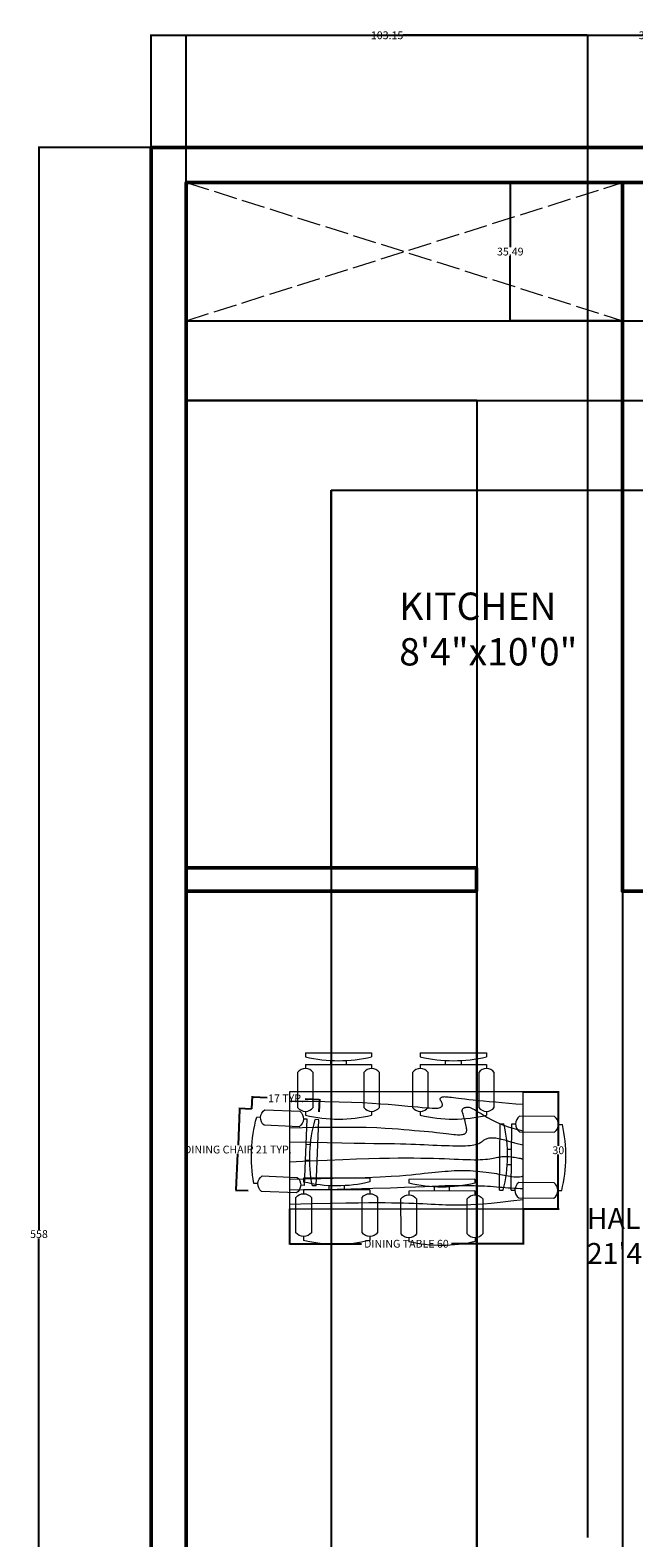
# Model space of a CAD drawing. Units: inches. Extents: x 32 to 429, y 30 to 648.
# Tile 2 of 3: x 32 to 187, y 261 to 648. Entities that reach past the tile are written whole.
import ezdxf

# ---------------------------------------------------------------- set-up
doc = ezdxf.new("R2010")
doc.units = ezdxf.units.IN
doc.header["$MEASUREMENT"] = 0
doc.linetypes.add('ACAD_ISO02W100', pattern=[15, 12, -3])
for name, color, linetype, lineweight in [('A-ANNO-DIMS', 2, 'Continuous', 18), ('A-AREA-IDEN', 7, 'Continuous', 25), ('A-FLOR-CASE', 32, 'Continuous', 25), ('A-FLOR-OVHD', 8, 'ACAD_ISO02W100', 18), ('A-FURN', 9, 'Continuous', 18), ('A-WALL', 7, 'Continuous', 50)]:
    doc.layers.add(name, color=color, linetype=linetype, lineweight=lineweight)
doc.styles.get("Standard").update_dxf_attribs({"font": 'arial.ttf'})
doc.dimstyles.get("Standard").update_dxf_attribs({"dimtxt": 2, "dimasz": 0.18, "dimexe": 0.18, "dimexo": 0.0625, "dimgap": 0.09, "dimtad": 0, "dimtih": 1, "dimtoh": 1, "dimrnd": 2, "dimzin": 0, "dimdsep": 46, "dimlunit": 3, "dimtxsty": 'Standard', "dimcen": 0.09, "dimadec": 0, "dimazin": 0, "dimtfac": 1, "dimtofl": 0, "dimtmove": 0, "dimatfit": 3, "dimfxl": 1, "dimtolj": 1, "dimtzin": 0, "dimarcsym": 0})

# ---------------------------------------------------------------- blocks, each defined once
blk = doc.blocks.new('Chair - Desk')
for p, q in [((-8.5, 0), (-8.5, -1)), ((-8.5, 0), (8.5, 0)), ((8.5, 0), (8.5, -1)), ((-8.5, -3), (-8.5, -4)), ((-8.5, -3), (8.5, -3)), ((-2, -3), (-2, -1.9355)), ((2, -1.9576), (2, -3)), ((8.5, -3), (8.5, -4)), ((-10.5, -5), (-10.5, -14)), ((-6.5, -14), (-6.5, -5)), ((6.5, -5), (6.5, -14)), ((10.5, -14), (10.5, -5)), ((-8.5, -15), (-8.5, -16)), ((8.5, -15), (8.5, -16))]:
    blk.add_line(p, q)
for centre, radius, start, end in [((0, 34.625), 36.625, 256.5803, 283.4197), ((-8.5, -6.5), 2.5, 36.8699, 143.1301), ((8.5, -6.5), 2.5, 36.8699, 143.1301), ((-8.5, -12.5), 2.5, 216.8699, 323.1301), ((8.5, -12.5), 2.5, 216.8699, 323.1301), ((0, 19.625), 36.625, 256.5803, 283.4197)]:
    blk.add_arc(centre, radius, start, end)
blk = doc.blocks.new('Table - Rectangular Woodgrain 60 x 30 in.')
for p, q in [((0, 0), (0, -30)), ((60, 0), (0, 0)), ((60, -30), (60, 0)), ((0, -30), (60, -30))]:
    blk.add_line(p, q)
for points in [[(0, -2.4), (4.8155, -2.418), (9.0302, -2.4688), (12.709, -2.5477), (15.9167, -2.65), (18.7181, -2.7711), (21.1781, -2.9063), (23.3616, -3.0508), (25.3333, -3.2), (27.1477, -3.3495), (28.8172, -3.4958), (30.3437, -3.636), (31.7291, -3.7667), (32.9756, -3.8849), (34.0849, -3.9875), (35.059, -4.0714), (35.9, -4.1334), (36.6114, -4.1711), (37.2041, -4.1854), (37.6906, -4.1779), (38.0833, -4.15), (38.3948, -4.1034), (38.6375, -4.0396), (38.8239, -3.9602), (38.9666, -3.8667), (39.0764, -3.7608), (39.1573, -3.6448), (39.2116, -3.521), (39.2416, -3.3917), (39.2498, -3.2593), (39.2385, -3.1261), (39.21, -2.9944), (39.1666, -2.8667), (39.111, -2.7447), (39.0468, -2.6281), (38.978, -2.5163), (38.9083, -2.4083), (38.8418, -2.3035), (38.7823, -2.201), (38.7337, -2.1001), (38.7, -2), (38.6844, -1.9003), (38.6875, -1.8021), (38.7094, -1.707), (38.75, -1.6167), (38.8094, -1.5326), (38.8875, -1.4563), (38.9844, -1.3893), (39.1, -1.3333), (39.2351, -1.2896), (39.3937, -1.2583), (39.5804, -1.2396), (39.8, -1.2333), (40.057, -1.2396), (40.3562, -1.2583), (40.7023, -1.2896), (41.1, -1.3333), (41.5547, -1.3895), (42.0755, -1.4573), (42.6721, -1.5361), (43.3542, -1.625), (44.1316, -1.7233), (45.014, -1.8302), (46.0114, -1.9449), (47.1333, -2.0667), (48.3862, -2.1947), (49.7625, -2.3281), (51.2513, -2.4663), (52.8416, -2.6083), (54.5226, -2.7535), (56.2833, -2.9011), (58.1127, -3.0501), (60, -3.2)], [(0, -9.2), (6.5759, -9.0858), (11.9385, -9.0365), (16.2527, -9.0418), (19.6833, -9.0917), (22.3952, -9.1759), (24.5531, -9.2844), (26.322, -9.4069), (27.8666, -9.5333), (29.3241, -9.6553), (30.7203, -9.7719), (32.0532, -9.8837), (33.3208, -9.9917), (34.5213, -10.0965), (35.6526, -10.199), (36.7128, -10.2999), (37.7, -10.4), (38.6129, -10.4996), (39.4531, -10.5969), (40.223, -10.6895), (40.925, -10.775), (41.5613, -10.8512), (42.1344, -10.9156), (42.6465, -10.966), (43.1, -11), (43.4976, -11.0158), (43.8437, -11.0136), (44.143, -10.9942), (44.4, -10.9583), (44.6195, -10.9069), (44.8062, -10.8406), (44.9648, -10.7603), (45.1, -10.6667), (45.2155, -10.5598), (45.3114, -10.4365), (45.3871, -10.2929), (45.4416, -10.125), (45.4743, -9.929), (45.4844, -9.7011), (45.4709, -9.4371), (45.4333, -9.1333), (45.3716, -8.7883), (45.2896, -8.4104), (45.1919, -8.0107), (45.0833, -7.6), (44.9685, -7.1893), (44.8521, -6.7896), (44.7388, -6.4117), (44.6333, -6.0667), (44.54, -5.7628), (44.4614, -5.4979), (44.4001, -5.2675), (44.3583, -5.0667), (44.3384, -4.8909), (44.3427, -4.7354), (44.3736, -4.5956), (44.4333, -4.4667), (44.5236, -4.3453), (44.6427, -4.2333), (44.7884, -4.1339), (44.9583, -4.05), (45.1501, -3.9849), (45.3614, -3.9417), (45.59, -3.9234), (45.8333, -3.9333), (46.0915, -3.9749), (46.3734, -4.0531), (46.6906, -4.1736), (47.0542, -4.3417), (47.4756, -4.5629), (47.9661, -4.8427), (48.5372, -5.1866), (49.2, -5.6), (49.9676, -6.0844), (50.8594, -6.625), (51.8965, -7.2031), (53.1, -7.8), (54.491, -8.3969), (56.0906, -8.975), (57.9199, -9.5156), (60, -10)], [(0, -12.8), (5.1847, -12.9322), (9.6213, -13.0323), (13.3963, -13.1059), (16.5958, -13.1583), (19.3063, -13.1952), (21.614, -13.2219), (23.6054, -13.2439), (25.3666, -13.2667), (26.9728, -13.2947), (28.4531, -13.3281), (29.8256, -13.3663), (31.1083, -13.4083), (32.3191, -13.4535), (33.476, -13.501), (34.597, -13.5501), (35.7, -13.6), (36.7984, -13.6497), (37.8875, -13.6979), (38.9578, -13.743), (40, -13.7833), (41.0047, -13.8174), (41.9625, -13.8438), (42.864, -13.8607), (43.7, -13.8667), (44.4631, -13.8604), (45.1552, -13.8417), (45.7801, -13.8104), (46.3416, -13.7667), (46.8439, -13.7104), (47.2906, -13.6417), (47.6858, -13.5604), (48.0333, -13.4667), (48.3375, -13.3608), (48.6042, -13.2448), (48.8396, -13.121), (49.05, -12.9917), (49.2417, -12.8593), (49.4208, -12.7261), (49.5937, -12.5944), (49.7667, -12.4667), (49.9452, -12.3451), (50.1323, -12.2313), (50.3303, -12.1268), (50.5416, -12.0333), (50.7686, -11.9524), (51.0135, -11.8854), (51.2788, -11.8341), (51.5666, -11.8), (51.8785, -11.7843), (52.2116, -11.7865), (52.562, -11.8059), (52.926, -11.8417), (53.2998, -11.8931), (53.6795, -11.9594), (54.0614, -12.0397), (54.4416, -12.1333), (54.8223, -12.2401), (55.2293, -12.3625), (55.6942, -12.5037), (56.2489, -12.6667), (56.9251, -12.8547), (57.7545, -13.0708), (58.7689, -13.3182), (60, -13.6)], [(0, -18), (5.124, -17.7273), (9.6609, -17.5057), (13.6705, -17.3303), (17.2125, -17.1958), (20.3467, -17.0973), (23.1328, -17.0297), (25.6307, -16.9878), (27.9, -16.9667), (29.9928, -16.9617), (31.9302, -16.9703), (33.7254, -16.9907), (35.3917, -17.0208), (36.9423, -17.0588), (38.3906, -17.1026), (39.7499, -17.1503), (41.0333, -17.2), (42.2519, -17.2496), (43.4073, -17.2969), (44.4986, -17.3395), (45.525, -17.375), (46.4858, -17.4012), (47.3802, -17.4156), (48.2074, -17.416), (48.9667, -17.4), (49.6583, -17.3662), (50.2872, -17.3167), (50.8595, -17.2547), (51.3812, -17.1833), (51.8584, -17.1057), (52.2971, -17.025), (52.7034, -16.9443), (53.0833, -16.8667), (53.443, -16.7951), (53.789, -16.7313), (54.128, -16.6768), (54.4666, -16.6334), (54.8115, -16.6024), (55.1693, -16.5854), (55.5465, -16.5841), (55.95, -16.6), (56.3828, -16.6337), (56.8346, -16.6823), (57.2915, -16.7418), (57.7396, -16.8084), (58.165, -16.878), (58.5539, -16.9469), (58.8924, -17.0111), (59.1666, -17.0667), (59.3679, -17.1107), (59.5078, -17.1438), (59.6032, -17.1675), (59.6708, -17.1833), (59.7275, -17.193), (59.7901, -17.1979), (59.8753, -17.1998), (60, -17.2)], [(0, -22.4), (8.0098, -22.2501), (14.4094, -22.1011), (19.4168, -21.9535), (23.25, -21.8083), (26.1269, -21.6663), (28.2656, -21.5281), (29.884, -21.3947), (31.2, -21.2667), (32.3967, -21.1448), (33.5172, -21.0292), (34.5697, -20.9198), (35.5625, -20.8167), (36.5037, -20.7198), (37.4015, -20.6292), (38.2642, -20.5448), (39.1, -20.4667), (39.9164, -20.3951), (40.7187, -20.3313), (41.5117, -20.2768), (42.3, -20.2333), (43.0883, -20.2024), (43.8812, -20.1854), (44.6836, -20.1841), (45.5, -20.2), (46.3328, -20.234), (47.1747, -20.2844), (48.0163, -20.3488), (48.8479, -20.425), (49.66, -20.5106), (50.4429, -20.6031), (51.1872, -20.7004), (51.8833, -20.8), (52.5246, -20.8999), (53.1166, -20.9995), (53.6681, -21.0983), (54.1875, -21.1958), (54.6834, -21.2919), (55.1646, -21.3859), (55.6394, -21.4777), (56.1167, -21.5667), (56.6028, -21.6515), (57.0961, -21.7266), (57.5929, -21.7852), (58.0896, -21.8208), (58.5823, -21.8268), (59.0674, -21.7964), (59.5412, -21.723), (60, -21.6)], [(0, -25.2), (8.6355, -25.0504), (15.7026, -24.9031), (21.4049, -24.7606), (25.9458, -24.625), (29.529, -24.4988), (32.3578, -24.3844), (34.6359, -24.284), (36.5667, -24.2), (38.3213, -24.1341), (39.9417, -24.0854), (41.437, -24.0523), (42.8167, -24.0333), (44.0901, -24.0268), (45.2667, -24.0313), (46.3557, -24.0451), (47.3667, -24.0667), (48.309, -24.0947), (49.1928, -24.1287), (50.0284, -24.168), (50.826, -24.2125), (51.5959, -24.2617), (52.3483, -24.3151), (53.0935, -24.3725), (53.8417, -24.4334), (54.6009, -24.497), (55.3699, -24.561), (56.1454, -24.6226), (56.9239, -24.6792), (57.7021, -24.7279), (58.4764, -24.7662), (59.2435, -24.7911), (60, -24.8)], [(0, -28.8), (5.6867, -28.6681), (10.45, -28.5698), (14.407, -28.5012), (17.675, -28.4584), (20.3711, -28.4374), (22.6125, -28.4344), (24.5164, -28.4455), (26.2, -28.4667), (27.762, -28.4947), (29.2276, -28.5281), (30.6033, -28.5663), (31.8958, -28.6084), (33.1118, -28.6535), (34.2578, -28.7011), (35.3405, -28.7501), (36.3666, -28.8), (37.3443, -28.8497), (38.288, -28.8974), (39.2137, -28.9412), (40.1375, -28.9792), (41.0753, -29.0093), (42.0432, -29.0297), (43.0572, -29.0384), (44.1333, -29.0333), (45.2936, -29.0114), (46.5843, -28.9641), (48.0579, -28.8816), (49.7666, -28.7542), (51.7629, -28.5721), (54.0989, -28.3255), (56.8272, -28.0048), (60, -27.6)]]:
    blk.add_lwpolyline(points)
blk = doc.blocks.new('*D21')
at = {"layer": 'A-ANNO-DIMS', "color": 0, "lineweight": -2, "transparency": 16777216}
for p, q in [((86.09, 371), (85.71, 361.81)), ((89.18, 371.05), (85.92, 371.19)), ((85.24, 350.38), (85.62, 359.56)), ((88.31, 350.07), (85.05, 350.2))]:
    blk.add_line(p, q, dxfattribs=at)
at = {"layer": 'A-ANNO-DIMS', "color": 0, "transparency": 16777216}
for points in [[(86.06, 371), (86.12, 371), (86.1, 371.18)], [(85.21, 350.38), (85.27, 350.38), (85.23, 350.2)]]:
    blk.add_solid(points, dxfattribs=at)
at = {"layer": 'Defpoints', "color": 0, "transparency": 16777216}
for p in [(86.1, 371.18), (89.24, 371.05), (88.38, 350.07)]:
    blk.add_point(p, dxfattribs=at)
at = {"layer": 'A-ANNO-DIMS', "color": 0, "transparency": 16777216, "insert": (85.66, 360.69), "char_height": 2, "attachment_point": 5}
blk.add_mtext('\\A1;DINING CHAIR 21 TYP.', dxfattribs=at)
blk = doc.blocks.new('*D22')
at = {"layer": 'A-ANNO-DIMS', "color": 0, "lineweight": -2, "transparency": 16777216}
for p, q in [((89.25, 371.11), (89.38, 374.38)), ((89.55, 374.19), (93.17, 374.04)), ((106.51, 373.49), (102.9, 373.64)), ((106.57, 370.4), (106.7, 373.66))]:
    blk.add_line(p, q, dxfattribs=at)
at = {"layer": 'A-ANNO-DIMS', "color": 0, "transparency": 16777216}
for points in [[(89.56, 374.22), (89.55, 374.16), (89.37, 374.2)], [(106.51, 373.52), (106.51, 373.46), (106.69, 373.48)]]:
    blk.add_solid(points, dxfattribs=at)
at = {"layer": 'Defpoints', "color": 0, "transparency": 16777216}
for p in [(106.69, 373.48), (89.24, 371.05), (106.56, 370.33)]:
    blk.add_point(p, dxfattribs=at)
at = {"layer": 'A-ANNO-DIMS', "color": 0, "transparency": 16777216, "insert": (98.03, 373.84), "char_height": 2, "attachment_point": 5}
blk.add_mtext('\\A1;17 TYP.', dxfattribs=at)
blk = doc.blocks.new('*D23')
at = {"layer": 'A-ANNO-DIMS', "color": 0, "lineweight": -2, "transparency": 16777216}
for p, q in [((98.93, 345.45), (98.93, 336.33)), ((158.93, 345.45), (158.93, 336.33)), ((99.11, 336.51), (117.37, 336.51)), ((158.75, 336.51), (140.49, 336.51))]:
    blk.add_line(p, q, dxfattribs=at)
at = {"layer": 'A-ANNO-DIMS', "color": 0, "transparency": 16777216}
for points in [[(99.11, 336.54), (99.11, 336.48), (98.93, 336.51)], [(158.75, 336.54), (158.75, 336.48), (158.93, 336.51)]]:
    blk.add_solid(points, dxfattribs=at)
at = {"layer": 'Defpoints', "color": 0, "transparency": 16777216}
for p in [(98.93, 345.51), (158.93, 345.51), (158.93, 336.51)]:
    blk.add_point(p, dxfattribs=at)
at = {"layer": 'A-ANNO-DIMS', "color": 0, "transparency": 16777216, "insert": (128.93, 336.51), "char_height": 2, "attachment_point": 5}
blk.add_mtext('\\A1;DINING TABLE 60', dxfattribs=at)
blk = doc.blocks.new('*D24')
at = {"layer": 'A-ANNO-DIMS', "color": 0, "lineweight": -2, "transparency": 16777216}
for p, q in [((158.99, 375.51), (168.11, 375.51)), ((167.93, 375.33), (167.93, 361.62)), ((167.93, 345.69), (167.93, 359.4)), ((158.99, 345.51), (168.11, 345.51))]:
    blk.add_line(p, q, dxfattribs=at)
at = {"layer": 'A-ANNO-DIMS', "color": 0, "transparency": 16777216}
for points in [[(167.9, 375.33), (167.96, 375.33), (167.93, 375.51)], [(167.9, 345.69), (167.96, 345.69), (167.93, 345.51)]]:
    blk.add_solid(points, dxfattribs=at)
at = {"layer": 'Defpoints', "color": 0, "transparency": 16777216}
for p in [(158.93, 375.51), (167.93, 375.51), (158.93, 345.51)]:
    blk.add_point(p, dxfattribs=at)
at = {"layer": 'A-ANNO-DIMS', "color": 0, "transparency": 16777216, "insert": (167.93, 360.51), "char_height": 2, "attachment_point": 5}
blk.add_mtext('\\A1;30', dxfattribs=at)
blk = doc.blocks.new('*D33')
at = {"layer": 'A-ANNO-DIMS', "color": 0, "lineweight": -2, "transparency": 16777216}
for p, q in [((63.39, 618.06), (63.39, 646.97)), ((63.57, 646.79), (202.09, 646.79)), ((345.21, 646.79), (206.7, 646.79)), ((345.39, 618.06), (345.39, 646.97))]:
    blk.add_line(p, q, dxfattribs=at)
at = {"layer": 'A-ANNO-DIMS', "color": 0, "transparency": 16777216}
for points in [[(63.57, 646.82), (63.57, 646.76), (63.39, 646.79)], [(345.21, 646.82), (345.21, 646.76), (345.39, 646.79)]]:
    blk.add_solid(points, dxfattribs=at)
at = {"layer": 'Defpoints', "color": 0, "transparency": 16777216}
for p in [(345.39, 646.79), (63.39, 617.99), (345.39, 617.99)]:
    blk.add_point(p, dxfattribs=at)
at = {"layer": 'A-ANNO-DIMS', "color": 0, "transparency": 16777216, "insert": (204.39, 646.79), "char_height": 2, "attachment_point": 5}
blk.add_mtext('\\A1;282', dxfattribs=at)
blk = doc.blocks.new('*D34')
at = {"layer": 'A-ANNO-DIMS', "color": 0, "lineweight": -2, "transparency": 16777216}
for p, q in [((63.33, 617.99), (34.41, 617.99)), ((34.59, 617.81), (34.59, 340.1)), ((34.59, 60.17), (34.59, 337.88)), ((63.33, 59.99), (34.41, 59.99))]:
    blk.add_line(p, q, dxfattribs=at)
at = {"layer": 'A-ANNO-DIMS', "color": 0, "transparency": 16777216}
for points in [[(34.56, 617.81), (34.62, 617.81), (34.59, 617.99)], [(34.56, 60.17), (34.62, 60.17), (34.59, 59.99)]]:
    blk.add_solid(points, dxfattribs=at)
at = {"layer": 'Defpoints', "color": 0, "transparency": 16777216}
for p in [(34.59, 617.99), (63.39, 617.99), (63.39, 59.99)]:
    blk.add_point(p, dxfattribs=at)
at = {"layer": 'A-ANNO-DIMS', "color": 0, "transparency": 16777216, "insert": (34.59, 338.99), "char_height": 2, "attachment_point": 5}
blk.add_mtext('\\A1;558', dxfattribs=at)
blk = doc.blocks.new('*D43')
at = {"layer": 'A-ANNO-DIMS', "color": 0, "lineweight": -2, "transparency": 16777216}
for p, q in [((72.39, 426.93), (72.39, 31.01)), ((146.89, 426.93), (146.89, 31.01)), ((72.57, 31.19), (106.96, 31.19)), ((146.71, 31.19), (112.33, 31.19))]:
    blk.add_line(p, q, dxfattribs=at)
at = {"layer": 'A-ANNO-DIMS', "color": 0, "transparency": 16777216}
for points in [[(72.57, 31.22), (72.57, 31.16), (72.39, 31.19)], [(146.71, 31.22), (146.71, 31.16), (146.89, 31.19)]]:
    blk.add_solid(points, dxfattribs=at)
at = {"layer": 'Defpoints', "color": 0, "transparency": 16777216}
for p in [(72.39, 426.99), (146.89, 426.99), (146.89, 31.19)]:
    blk.add_point(p, dxfattribs=at)
at = {"layer": 'A-ANNO-DIMS', "color": 0, "transparency": 16777216, "insert": (109.64, 31.19), "char_height": 2, "attachment_point": 5}
blk.add_mtext('\\A1;74.5', dxfattribs=at)
blk = doc.blocks.new('*D44')
at = {"layer": 'A-ANNO-DIMS', "color": 0, "lineweight": -2, "transparency": 16777216}
for p, q in [((146.89, 426.93), (146.89, 31.01)), ((184.39, 426.93), (184.39, 31.01)), ((147.07, 31.19), (162.95, 31.19)), ((184.21, 31.19), (168.34, 31.19))]:
    blk.add_line(p, q, dxfattribs=at)
at = {"layer": 'A-ANNO-DIMS', "color": 0, "transparency": 16777216}
for points in [[(147.07, 31.22), (147.07, 31.16), (146.89, 31.19)], [(184.21, 31.22), (184.21, 31.16), (184.39, 31.19)]]:
    blk.add_solid(points, dxfattribs=at)
at = {"layer": 'Defpoints', "color": 0, "transparency": 16777216}
for p in [(146.89, 426.99), (184.39, 426.99), (184.39, 31.19)]:
    blk.add_point(p, dxfattribs=at)
at = {"layer": 'A-ANNO-DIMS', "color": 0, "transparency": 16777216, "insert": (165.64, 31.19), "char_height": 2, "attachment_point": 5}
blk.add_mtext('\\A1;37.5', dxfattribs=at)
blk = doc.blocks.new('*D46')
at = {"layer": 'A-ANNO-DIMS', "color": 0, "lineweight": -2, "transparency": 16777216}
for p, q in [((175.55, 261.06), (175.55, 646.97)), ((175.73, 646.79), (188.5, 646.79)), ((208.21, 646.79), (195.44, 646.79)), ((208.39, 261.06), (208.39, 646.97))]:
    blk.add_line(p, q, dxfattribs=at)
at = {"layer": 'A-ANNO-DIMS', "color": 0, "transparency": 16777216}
for points in [[(175.73, 646.82), (175.73, 646.76), (175.55, 646.79)], [(208.21, 646.82), (208.21, 646.76), (208.39, 646.79)]]:
    blk.add_solid(points, dxfattribs=at)
at = {"layer": 'Defpoints', "color": 0, "transparency": 16777216}
for p in [(208.39, 646.79), (175.55, 260.99), (208.39, 260.99)]:
    blk.add_point(p, dxfattribs=at)
at = {"layer": 'A-ANNO-DIMS', "color": 0, "transparency": 16777216, "insert": (191.97, 646.79), "char_height": 2, "attachment_point": 5}
blk.add_mtext('\\A1;32.85', dxfattribs=at)
blk = doc.blocks.new('*D49')
at = {"layer": 'A-ANNO-DIMS', "color": 0, "lineweight": -2, "transparency": 16777216}
for p, q in [((109.64, 529.9), (109.64, 31.01)), ((147.02, 529.9), (147.02, 31.01)), ((109.82, 31.19), (124.08, 31.19)), ((146.84, 31.19), (132.58, 31.19))]:
    blk.add_line(p, q, dxfattribs=at)
at = {"layer": 'A-ANNO-DIMS', "color": 0, "transparency": 16777216}
for points in [[(109.82, 31.22), (109.82, 31.16), (109.64, 31.19)], [(146.84, 31.22), (146.84, 31.16), (147.02, 31.19)]]:
    blk.add_solid(points, dxfattribs=at)
at = {"layer": 'Defpoints', "color": 0, "transparency": 16777216}
for p in [(109.64, 529.96), (147.02, 529.96), (147.02, 31.19)]:
    blk.add_point(p, dxfattribs=at)
at = {"layer": 'A-ANNO-DIMS', "color": 0, "transparency": 16777216, "insert": (128.33, 31.19), "char_height": 2, "attachment_point": 5}
blk.add_mtext('\\A1;37.375', dxfattribs=at)
blk = doc.blocks.new('*D50')
at = {"layer": 'A-ANNO-DIMS', "color": 0, "lineweight": -2, "transparency": 16777216}
for p, q in [((147.08, 552.99), (425.41, 552.99)), ((425.23, 552.81), (425.23, 542.59)), ((425.23, 530.14), (425.23, 540.36)), ((147.08, 529.96), (425.41, 529.96))]:
    blk.add_line(p, q, dxfattribs=at)
at = {"layer": 'A-ANNO-DIMS', "color": 0, "transparency": 16777216}
for points in [[(425.2, 552.81), (425.26, 552.81), (425.23, 552.99)], [(425.2, 530.14), (425.26, 530.14), (425.23, 529.96)]]:
    blk.add_solid(points, dxfattribs=at)
at = {"layer": 'Defpoints', "color": 0, "transparency": 16777216}
for p in [(147.02, 552.99), (147.02, 529.96), (425.23, 529.96)]:
    blk.add_point(p, dxfattribs=at)
at = {"layer": 'A-ANNO-DIMS', "color": 0, "transparency": 16777216, "insert": (425.23, 541.48), "char_height": 2, "attachment_point": 5}
blk.add_mtext('\\A1;23.034', dxfattribs=at)
blk = doc.blocks.new('*D53')
at = {"layer": 'A-ANNO-DIMS', "color": 0, "lineweight": -2, "transparency": 16777216}
for p, q in [((72.39, 261.06), (72.39, 646.97)), ((72.57, 646.79), (119.82, 646.79)), ((175.37, 646.79), (128.13, 646.79)), ((175.55, 261.06), (175.55, 646.97))]:
    blk.add_line(p, q, dxfattribs=at)
at = {"layer": 'A-ANNO-DIMS', "color": 0, "transparency": 16777216}
for points in [[(72.57, 646.82), (72.57, 646.76), (72.39, 646.79)], [(175.37, 646.82), (175.37, 646.76), (175.55, 646.79)]]:
    blk.add_solid(points, dxfattribs=at)
at = {"layer": 'Defpoints', "color": 0, "transparency": 16777216}
for p in [(175.55, 646.79), (72.39, 260.99), (175.55, 260.99)]:
    blk.add_point(p, dxfattribs=at)
at = {"layer": 'A-ANNO-DIMS', "color": 0, "transparency": 16777216, "insert": (123.97, 646.79), "char_height": 2, "attachment_point": 5}
blk.add_mtext('\\A1;103.15', dxfattribs=at)
blk = doc.blocks.new('*D55')
at = {"layer": 'A-ANNO-DIMS', "color": 0, "lineweight": -2, "transparency": 16777216}
for p, q in [((184.33, 608.99), (155.41, 608.99)), ((155.59, 608.81), (155.59, 592.36)), ((155.59, 573.68), (155.59, 590.14)), ((184.33, 573.5), (155.41, 573.5))]:
    blk.add_line(p, q, dxfattribs=at)
at = {"layer": 'A-ANNO-DIMS', "color": 0, "transparency": 16777216}
for points in [[(155.56, 608.81), (155.62, 608.81), (155.59, 608.99)], [(155.56, 573.68), (155.62, 573.68), (155.59, 573.5)]]:
    blk.add_solid(points, dxfattribs=at)
at = {"layer": 'Defpoints', "color": 0, "transparency": 16777216}
for p in [(155.59, 608.99), (184.39, 608.99), (184.39, 573.5)]:
    blk.add_point(p, dxfattribs=at)
at = {"layer": 'A-ANNO-DIMS', "color": 0, "transparency": 16777216, "insert": (155.59, 591.25), "char_height": 2, "attachment_point": 5}
blk.add_mtext('\\A1;35.49', dxfattribs=at)
blk = doc.blocks.new('*D56')
at = {"layer": 'A-ANNO-DIMS', "color": 0, "lineweight": -2, "transparency": 16777216}
for p, q in [((72.46, 573.5), (425.41, 573.5)), ((425.23, 573.32), (425.23, 564.36)), ((425.23, 553.17), (425.23, 562.14)), ((72.46, 552.99), (425.41, 552.99))]:
    blk.add_line(p, q, dxfattribs=at)
at = {"layer": 'A-ANNO-DIMS', "color": 0, "transparency": 16777216}
for points in [[(425.2, 573.32), (425.26, 573.32), (425.23, 573.5)], [(425.2, 553.17), (425.26, 553.17), (425.23, 552.99)]]:
    blk.add_solid(points, dxfattribs=at)
at = {"layer": 'Defpoints', "color": 0, "transparency": 16777216}
for p in [(72.39, 573.5), (425.23, 573.5), (72.39, 552.99)]:
    blk.add_point(p, dxfattribs=at)
at = {"layer": 'A-ANNO-DIMS', "color": 0, "transparency": 16777216, "insert": (425.23, 563.25), "char_height": 2, "attachment_point": 5}
blk.add_mtext('\\A1;20.51', dxfattribs=at)

msp = doc.modelspace()

# ---------------------------------------------------------------- linework, layer by layer
at = {"layer": 'A-FLOR-CASE'}
for p, q in [((147.0192, 552.9929), (72.3942, 552.9929)), ((147.0192, 552.9929), (147.0192, 529.9584)), ((109.6441, 432.9929), (109.6441, 529.9584)), ((109.6441, 529.9584), (147.0192, 529.9584))]:
    msp.add_line(p, q, dxfattribs=at)
at = {"layer": 'A-FLOR-OVHD', "ltscale": 0.5}
for p, q in [((72.3942, 608.9929), (184.3942, 573.5041)), ((72.3942, 573.5041), (184.3942, 608.9929)), ((72.3942, 573.5041), (184.3942, 573.5041))]:
    msp.add_line(p, q, dxfattribs=at)
at = {"layer": 'A-WALL'}
msp.add_line((72.3942, 608.9929), (172.3942, 608.9929), dxfattribs=at)
for points in [[(208.3942, 59.9929), (345.3942, 59.9929), (345.3942, 617.9929), (63.3942, 617.9929), (63.3942, 59.9929)], [(248.394, 254.9928), (248.394, 260.9928), (336.394, 260.9928), (336.394, 608.9928), (72.394, 608.9928), (72.394, 59.9928)], [(336.3942, 608.9929), (184.3942, 608.9929), (184.3942, 432.9929), (184.3942, 426.9929), (190.3942, 426.9929), (190.3942, 608.9929)], [(72.3942, 432.9929), (146.8939, 432.9929), (146.8939, 426.9929), (72.3942, 426.9929)]]:
    msp.add_lwpolyline(points, dxfattribs=at)

# ---------------------------------------------------------------- block references
at = {"layer": 'A-FURN'}
for name, p in [('Chair - Desk', (111.5, 385.5)), ('Chair - Desk', (141, 385.5)), ('Table - Rectangular Woodgrain 60 x 30 in.', (98.9264, 375.5086))]:
    msp.add_blockref(name, p, dxfattribs=at)
at = {"layer": 'A-FURN', "xscale": -1}
for p, rotation in [((106.1291, 359.8423), 267.6339504191041), ((111.0297, 353.3538), 0.0487930957746485), ((138.0281, 353.0419), 0.0487930957746485)]:
    msp.add_blockref('Chair - Desk', p, dxfattribs=dict(at, rotation=rotation))
at = {"layer": 'A-FURN', "rotation": 89.44481550255745}
msp.add_blockref('Chair - Desk', (152.8849, 358.8046), dxfattribs=at)

# ---------------------------------------------------------------- texts
at = {"layer": 'A-AREA-IDEN', "insert": (127.0778, 503.7023), "char_height": 7.01794, "attachment_point": 1}
msp.add_mtext('KITCHEN\\P8\'4"x10\'0"', dxfattribs=at)
at = {"layer": 'A-AREA-IDEN', "insert": (175.2397, 345.6521), "char_height": 5.366729, "attachment_point": 1}
msp.add_mtext_dynamic_manual_height_columns('HALL\\P21\'4"X12\'8"', width=49.260324, gutter_width=26.8336, heights=[0], dxfattribs=at)

# ---------------------------------------------------------------- dimensions: what is measured, and where the dimension line sits
at = {"layer": 'A-ANNO-DIMS'}
for base, p1, p2, override, picture, middle in [((345.3942, 646.7929), (63.3942, 617.9929), (345.3942, 617.9929), {"dimdec": 0, "dimlfac": 1, "dimrnd": 0, "dimzin": 0, "dimdsep": 46, "dimlunit": 2}, '*D33', (204.3942, 646.7929)), ((175.5464, 646.7929), (72.3942, 260.9929), (175.5464, 260.9929), {"dimdec": 2, "dimlfac": 1, "dimrnd": 0, "dimzin": 0, "dimdsep": 46, "dimlunit": 2}, '*D53', (123.9703, 646.7929)), ((208.3942, 646.7929), (175.5464, 260.9929), (208.3942, 260.9929), {"dimdec": 2, "dimlfac": 1, "dimrnd": 0, "dimzin": 0, "dimdsep": 46, "dimlunit": 2}, '*D46', (191.9703, 646.7929)), ((147.0192, 31.1928), (109.6441, 529.9584), (147.0192, 529.9584), {"dimdec": 3, "dimlfac": 1, "dimrnd": 0, "dimzin": 0, "dimdsep": 46, "dimlunit": 2}, '*D49', (128.3316, 31.1928)), ((146.8939, 31.1928), (72.3942, 426.9929), (146.8939, 426.9929), {"dimdec": 1, "dimlfac": 1, "dimrnd": 0, "dimzin": 0, "dimdsep": 46, "dimlunit": 2}, '*D43', (109.6441, 31.1928)), ((184.3942, 31.1928), (146.8939, 426.9929), (184.3942, 426.9929), {"dimdec": 1, "dimlfac": 1, "dimrnd": 0, "dimzin": 0, "dimdsep": 46, "dimlunit": 2}, '*D44', (165.6441, 31.1928))]:
    dim = msp.add_linear_dim(base=base, p1=p1, p2=p2, dimstyle='Standard', override=override, dxfattribs=at)
    dim.commit()
    dim.dimension.update_dxf_attribs({"geometry": picture, "text_midpoint": middle})
for base, p1, p2, override, picture, middle in [((34.5942, 617.9929), (63.3942, 59.9929), (63.3942, 617.9929), {"dimdec": 0, "dimlfac": 1, "dimrnd": 0, "dimzin": 0, "dimdsep": 46, "dimlunit": 2}, '*D34', (34.5942, 338.9929)), ((155.5942, 608.9929), (184.3942, 573.5041), (184.3942, 608.9929), {"dimdec": 2, "dimlfac": 1, "dimrnd": 0, "dimzin": 0, "dimdsep": 46, "dimlunit": 2}, '*D55', (155.5942, 591.2485)), ((425.2284, 573.5041), (72.3942, 552.9929), (72.3942, 573.5041), {"dimdec": 2, "dimlfac": 1, "dimrnd": 0, "dimzin": 0, "dimdsep": 46, "dimlunit": 2}, '*D56', (425.2284, 563.2485)), ((425.22842, 529.95843), (147.01917, 552.99291), (147.01917, 529.95843), {"dimdec": 3, "dimlfac": 1, "dimrnd": 0, "dimzin": 0, "dimdsep": 46, "dimlunit": 2}, '*D50', (425.22842, 541.47567)), ((167.9264, 375.5086), (158.9264, 345.5086), (158.9264, 375.5086), {"dimdec": 0, "dimlfac": 1, "dimrnd": 0, "dimzin": 0, "dimdsep": 46, "dimlunit": 2}, '*D24', (167.9264, 360.5086))]:
    dim = msp.add_linear_dim(base=base, p1=p1, p2=p2, angle=90, dimstyle='Standard', override=override, dxfattribs=at)
    dim.commit()
    dim.dimension.update_dxf_attribs({"geometry": picture, "text_midpoint": middle})
for base, p1, p2, angle, text, picture, middle in [((106.6927, 373.4807), (89.2441, 371.0489), (106.5626, 370.3334), 357.63395, '<> TYP.', '*D22', (98.0334, 373.8385)), ((86.0968, 371.179), (88.3771, 350.0668), (89.2441, 371.0489), 87.63395, 'DINING CHAIR <> TYP.', '*D21', (85.6633, 360.6879))]:
    dim = msp.add_linear_dim(base=base, p1=p1, p2=p2, angle=angle, text=text, dimstyle='Standard', override={"dimdec": 0, "dimlfac": 1, "dimrnd": 0, "dimzin": 0, "dimdsep": 46, "dimlunit": 2}, dxfattribs=at)
    dim.commit()
    dim.dimension.update_dxf_attribs({"geometry": picture, "text_midpoint": middle})
dim = msp.add_linear_dim(base=(158.9264, 336.5086), p1=(98.9264, 345.5086), p2=(158.9264, 345.5086), text='DINING TABLE <>', dimstyle='Standard', override={"dimdec": 0, "dimlfac": 1, "dimrnd": 0, "dimzin": 0, "dimdsep": 46, "dimlunit": 2}, dxfattribs=at)
dim.commit()
dim.dimension.update_dxf_attribs({"geometry": '*D23', "text_midpoint": (128.9264, 336.5086)})

doc.saveas('drawing.dxf')
